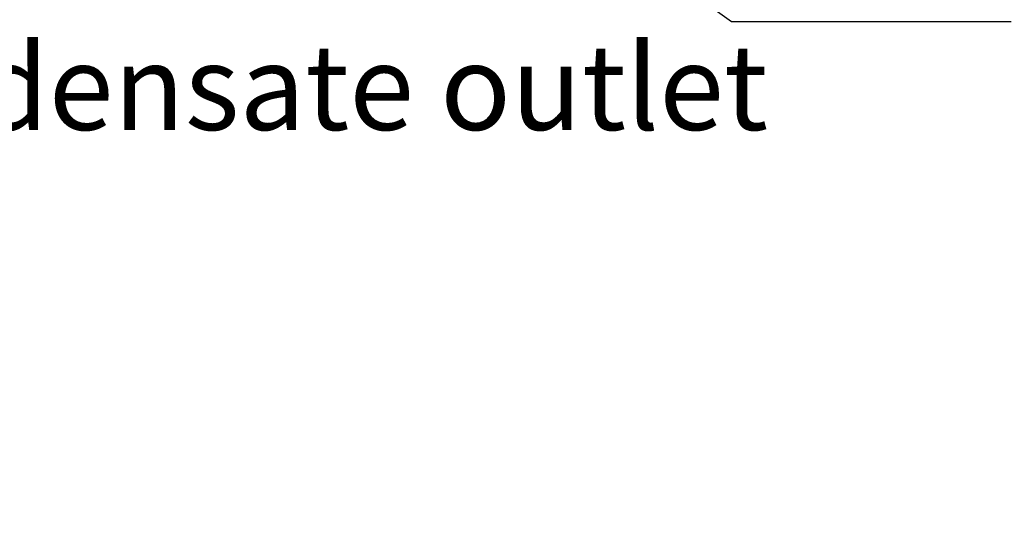
# Model space of a CAD drawing. Units: inches. Extents: x -12 to 334, y -10 to 186.
# Tile 29 of 77: x 106 to 152, y -10 to 14. Entities that reach past the tile are written whole.
import ezdxf
from ezdxf import colors
from ezdxf.entities.mleader import LeaderData, LeaderLine
from ezdxf.math import Vec2, Vec3

# ---------------------------------------------------------------- set-up
doc = ezdxf.new("R2010")
doc.units = ezdxf.units.IN
doc.header["$MEASUREMENT"] = 0
doc.layers.add('M-ANNO-TEXT', color=3, linetype='Continuous', lineweight=25)
doc.styles.get("Standard").update_dxf_attribs({"font": 'arial.ttf'})

msp = doc.modelspace()

# ---------------------------------------------------------------- leaders
at = {"layer": 'M-ANNO-TEXT'}
ml = msp.add_multileader_mtext('Standard', dxfattribs=at)
ml.set_content('^ICondensate outlet', color=256)
ml.set_leader_properties()
ml.build(insert=Vec2(0, 0))
ml.multileader.update_dxf_attribs({"dogleg_length": 0.36, "arrow_head_size": 0.7})
ctx = ml.context
ctx.base_point, ctx.arrow_head_size, ctx.landing_gap_size, ctx.plane_origin = Vec3(83.8784, 10.3512), 0.7, 0.09, Vec3(49.4251, 25.7584)
notes = []
notes.append((ctx, [(0, (1, 1, 0), (70.8242, 10.3512), (1, 0), 13.0542, [(0, [(42.9275, 33.6752)], 0, [])])]))
ctx.mtext.insert, ctx.mtext.flow_direction = Vec3(83.9684, 12.3853), 5
ml = msp.add_multileader_mtext('Standard', dxfattribs=at)
ml.set_content('liquid feed from\\Pcolumn', color=256)
ml.set_leader_properties()
ml.build(insert=Vec2(0, 0))
ml.multileader.update_dxf_attribs({"dogleg_length": 0.36, "arrow_head_size": 0.7})
ctx = ml.context
ctx.base_point, ctx.arrow_head_size, ctx.landing_gap_size, ctx.plane_origin = Vec3(152.1867, 13.4469), 0.7, 0.09, Vec3(117.7335, 28.8541)
notes.append((ctx, [(0, (1, 1, 0), (139.1325, 13.4469), (1, 0), 13.0542, [(0, [(117.7335, 28.8541)], 0, [])])]))
ctx.mtext.insert, ctx.mtext.flow_direction = Vec3(152.2767, 15.4796), 5
for ctx, leaders in notes:
    for number, flags, end, landing, length, lines in leaders:
        leader = LeaderData()
        leader.index, (leader.has_last_leader_line, leader.has_dogleg_vector, leader.attachment_direction) = number, flags
        leader.last_leader_point, leader.dogleg_vector, leader.dogleg_length = Vec3(end), Vec3(landing), length
        for number, points, colour, breaks in lines:
            line = LeaderLine()
            line.index, line.vertices, line.color, line.breaks = number, Vec3.list(points), colors.encode_raw_color(colour), breaks
            leader.lines.append(line)
        ctx.leaders.append(leader)

doc.saveas('drawing.dxf')
